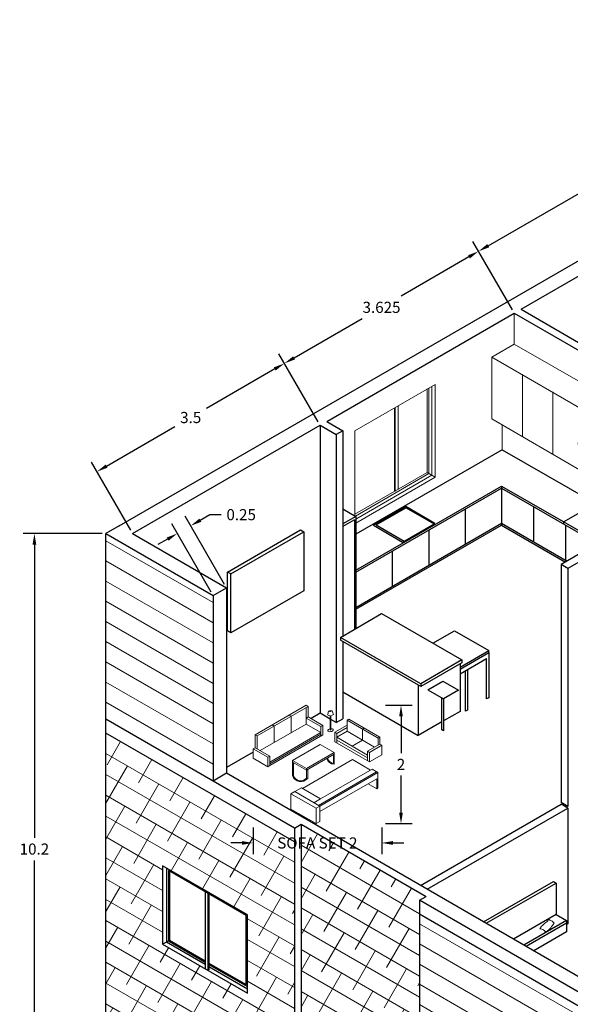
# Model space of a CAD drawing. Units: metres. Extents: x 14054 to 28215, y 4175 to 8383.
# Tile 2 of 6: x 14054.38 to 14063.29, y 4183.08 to 4199. Entities that reach past the tile are written whole.
import ezdxf

# ---------------------------------------------------------------- set-up
doc = ezdxf.new("R2010")
doc.units = ezdxf.units.M
for name, color, linetype, lineweight in [('A-ANNO-DIMS', 2, 'Continuous', 18), ('A-ANNO-NPLT', 9, 'Continuous', 13), ('A-ELEV-ISOM', 7, 'Continuous', 25), ('A-FURN', 8, 'Continuous', 13), ('A-GLAZ', 4, 'Continuous', 18), ('A-WALL-PATT', 8, 'Continuous', 13)]:
    doc.layers.add(name, color=color, linetype=linetype, lineweight=lineweight)
doc.styles.get("Standard").update_dxf_attribs({"font": 'arial.ttf'})
doc.dimstyles.get("Standard").update_dxf_attribs({"dimtxt": 0.18, "dimasz": 0.18, "dimexe": 0.18, "dimexo": 0.0625, "dimgap": 0.09, "dimtad": 0, "dimtih": 1, "dimtoh": 1, "dimdec": 4, "dimzin": 0, "dimdsep": 46, "dimtxsty": 'Standard', "dimcen": 0.09, "dimadec": 0, "dimazin": 0, "dimtfac": 1, "dimtdec": 4, "dimtofl": 0, "dimtmove": 0, "dimatfit": 3, "dimfxl": 1, "dimtolj": 1, "dimtzin": 0, "dimarcsym": 0})

# ---------------------------------------------------------------- blocks, each defined once
blk = doc.blocks.new('WINDOWS')
for p, q in [((14062.382, 4194.254), (14062.382, 4193.754)), ((14062.382, 4193.754), (14062.017, 4193.543)), ((14062.382, 4193.754), (14065.846, 4191.754)), ((14062.017, 4193.543), (14065.481, 4191.543)), ((14062.017, 4193.543), (14062.017, 4192.543)), ((14062.512, 4193.258), (14062.512, 4192.258)), ((14063.007, 4192.972), (14063.007, 4191.972)), ((14063.502, 4192.686), (14063.502, 4192.214)), ((14062.017, 4192.543), (14063.502, 4191.686)), ((14062.187, 4192.446), (14062.187, 4192.046)), ((14063.997, 4192.4), (14063.997, 4191.928)), ((14063.502, 4192.214), (14063.414, 4192.164)), ((14063.414, 4192.164), (14064.411, 4191.589)), ((14063.414, 4192.164), (14063.414, 4192.132)), ((14063.502, 4192.214), (14064.498, 4191.639)), ((14063.414, 4192.132), (14064.411, 4191.557)), ((14063.502, 4192.082), (14063.502, 4191.686)), ((14064.498, 4192.111), (14064.498, 4191.111)), ((14064.987, 4191.829), (14064.987, 4191.258)), ((14064.498, 4191.639), (14064.411, 4191.589)), ((14064.411, 4191.589), (14064.411, 4191.557)), ((14064.411, 4191.557), (14064.498, 4191.589)), ((14064.498, 4191.111), (14064.615, 4191.043))]:
    blk.add_line(p, q)
for p in [(14062.512, 4193.258), (14063.007, 4192.972), (14063.502, 4192.686), (14064.492, 4192.115), (14064.987, 4191.829)]:
    blk.add_point(p)
blk = doc.blocks.new('WINDOW')
for p, q in [((14059.806, 4192.353), (14061.105, 4193.103)), ((14061.105, 4193.103), (14061.105, 4191.603)), ((14060.975, 4193.028), (14060.975, 4191.678)), ((14061.002, 4193.043), (14061.002, 4191.663)), ((14061.047, 4193.069), (14061.047, 4191.637)), ((14060.445, 4192.722), (14060.445, 4191.384)), ((14060.456, 4192.728), (14060.456, 4191.378)), ((14060.505, 4192.756), (14060.505, 4191.406)), ((14059.806, 4190.976), (14059.806, 4192.353)), ((14060.975, 4191.678), (14059.806, 4191.003)), ((14060.975, 4191.678), (14061.105, 4191.603)), ((14061.002, 4191.663), (14059.815, 4190.971)), ((14061.047, 4191.637), (14059.821, 4190.923)), ((14061.105, 4191.603), (14059.821, 4190.861)), ((14060.456, 4191.378), (14060.445, 4191.384))]:
    blk.add_line(p, q)
blk = doc.blocks.new('SOFA SET')
for p, q in [((14050.583, 4183.453), (14052.129, 4184.345)), ((14050.646, 4183.417), (14052.188, 4184.311)), ((14052.129, 4184.345), (14052.188, 4184.311)), ((14052.129, 4183.775), (14052.129, 4184.277)), ((14052.188, 4183.991), (14052.188, 4184.311)), ((14052.841, 4184.171), (14052.866, 4184.172)), ((14052.841, 4184.171), (14052.841, 4184.156)), ((14052.866, 4184.172), (14052.866, 4184.158)), ((14051.674, 4184.013), (14051.614, 4184.048)), ((14051.674, 4184.013), (14051.674, 4183.512)), ((14052.129, 4183.957), (14052.188, 4183.991)), ((14052.572, 4183.701), (14052.129, 4183.957)), ((14052.631, 4183.735), (14052.188, 4183.991)), ((14052.851, 4183.602), (14052.851, 4184.028)), ((14052.868, 4183.603), (14052.868, 4184.029)), ((14053.361, 4183.896), (14053.411, 4183.925)), ((14054.298, 4183.355), (14053.361, 4183.896)), ((14053.361, 4183.896), (14053.361, 4183.56)), ((14054.348, 4183.384), (14053.411, 4183.925)), ((14052.129, 4183.775), (14050.741, 4182.974)), ((14051.16, 4183.715), (14051.099, 4183.75)), ((14051.16, 4183.715), (14051.16, 4183.216)), ((14052.129, 4183.775), (14052.572, 4183.519)), ((14052.572, 4183.701), (14052.631, 4183.735)), ((14052.572, 4183.416), (14052.572, 4183.701)), ((14052.572, 4183.622), (14052.572, 4183.416)), ((14052.631, 4183.735), (14052.631, 4183.45)), ((14052.989, 4183.528), (14053.361, 4183.743)), ((14053.048, 4183.494), (14053.361, 4183.675)), ((14053.048, 4183.379), (14053.361, 4183.56)), ((14053.361, 4183.56), (14054.193, 4183.079)), ((14053.83, 4183.626), (14053.879, 4183.654)), ((14053.83, 4183.289), (14053.83, 4183.626)), ((14050.583, 4183.064), (14050.583, 4183.453)), ((14050.583, 4183.453), (14050.646, 4183.417)), ((14050.646, 4183.028), (14050.646, 4183.417)), ((14051.027, 4182.627), (14052.572, 4183.519)), ((14052.572, 4183.469), (14051.027, 4182.577)), ((14051.027, 4182.524), (14052.631, 4183.45)), ((14052.572, 4183.416), (14052.631, 4183.45)), ((14052.989, 4183.528), (14052.989, 4183.243)), ((14052.989, 4183.528), (14053.048, 4183.494)), ((14053.048, 4183.494), (14053.048, 4183.209)), ((14053.048, 4183.379), (14053.98, 4182.841)), ((14053.048, 4183.292), (14053.98, 4182.754)), ((14053.83, 4183.289), (14053.516, 4183.109)), ((14054.298, 4183.355), (14054.348, 4183.384)), ((14054.298, 4183.355), (14054.298, 4183.14)), ((14054.348, 4183.169), (14054.348, 4183.384)), ((14050.524, 4183.03), (14050.583, 4183.064)), ((14050.968, 4182.775), (14050.524, 4183.03)), ((14050.524, 4182.746), (14050.524, 4183.03)), ((14051.027, 4182.808), (14050.583, 4183.064)), ((14051.717, 4182.68), (14052.549, 4183.161)), ((14052.549, 4183.161), (14052.968, 4182.919)), ((14052.989, 4183.243), (14054.039, 4182.637)), ((14053.98, 4182.956), (14054.348, 4183.169)), ((14054.039, 4182.922), (14054.406, 4183.135)), ((14054.348, 4183.169), (14054.406, 4183.135)), ((14054.406, 4183.135), (14054.406, 4182.85)), ((14050.524, 4182.746), (14050.968, 4182.49)), ((14050.968, 4182.775), (14051.027, 4182.808)), ((14050.968, 4182.49), (14050.968, 4182.775)), ((14051.027, 4182.808), (14051.027, 4182.524)), ((14051.717, 4182.68), (14052.136, 4182.438)), ((14051.717, 4182.68), (14051.717, 4182.629)), ((14052.014, 4181.835), (14053.522, 4182.706)), ((14052.968, 4182.919), (14052.136, 4182.438)), ((14052.968, 4182.868), (14052.136, 4182.387)), ((14052.95, 4182.857), (14052.95, 4182.587)), ((14052.968, 4182.919), (14052.968, 4182.868)), ((14052.968, 4182.868), (14052.968, 4182.571)), ((14054.07, 4182.389), (14053.522, 4182.706)), ((14053.98, 4182.956), (14053.98, 4182.671)), ((14053.98, 4182.956), (14054.039, 4182.922)), ((14054.039, 4182.922), (14054.039, 4182.637)), ((14054.039, 4182.637), (14054.406, 4182.85)), ((14050.968, 4182.49), (14051.027, 4182.524)), ((14051.717, 4182.629), (14052.136, 4182.387)), ((14051.717, 4182.629), (14051.717, 4182.222)), ((14051.747, 4182.612), (14051.747, 4182.23)), ((14052.136, 4182.438), (14052.136, 4182.387)), ((14052.136, 4182.387), (14052.136, 4182.145)), ((14052.173, 4182.408), (14052.173, 4182.138)), ((14052.563, 4181.519), (14054.115, 4182.415)), ((14054.115, 4182.415), (14054.295, 4182.311)), ((14052.498, 4181.322), (14054.253, 4182.335)), ((14052.54, 4181.297), (14054.295, 4182.311)), ((14054.259, 4182.128), (14052.54, 4181.136)), ((14054.259, 4181.827), (14054.259, 4182.128)), ((14054.295, 4182.311), (14054.295, 4181.848)), ((14051.982, 4181.854), (14051.78, 4181.737)), ((14051.982, 4181.854), (14052.563, 4181.519)), ((14054.259, 4181.827), (14053.998, 4181.977)), ((14054.295, 4181.848), (14054.259, 4181.827)), ((14051.669, 4181.673), (14051.78, 4181.737)), ((14052.43, 4181.234), (14051.669, 4181.673)), ((14051.669, 4181.673), (14051.669, 4181.21)), ((14052.54, 4181.297), (14051.78, 4181.737)), ((14052.563, 4181.519), (14052.36, 4181.401)), ((14052.43, 4180.771), (14051.669, 4181.21)), ((14052.54, 4181.297), (14052.43, 4181.234)), ((14052.43, 4181.234), (14052.43, 4180.771)), ((14052.54, 4181.297), (14052.54, 4180.835)), ((14052.54, 4180.835), (14052.43, 4180.771))]:
    blk.add_line(p, q)
for centre, radius, start, end in [((14051.304, 4184.571), 1.554, 340.4218, 344.7864), ((14052.864, 4184.075), 0.107, 65.1675, 123.9082), ((14052.847, 4184.288), 0.132, 251.1123, 297.9633), ((14053.99, 4184.575), 1.155, 200.4581, 206.1076), ((14052.85, 4184.184), 0.156, 238.6818, 311.6356), ((14052.859, 4183.606), 0.00924, 209.3503, 340.6112), ((14052.959, 4182.785), 0.215, 191.8594, 272.3236), ((14052.98, 4182.8), 0.215, 192.442, 261.974), ((14051.968, 4182.306), 0.265, 198.4938, 320.7512), ((14051.963, 4182.286), 0.224, 194.5089, 320.6289)]:
    blk.add_arc(centre, radius, start, end)
blk.add_ellipse((14052.863, 4183.591), major_axis=(0.0831, 0.0164), ratio=0.501593, start_param=1.613506, end_param=7.695336)
for p in [(14051.674, 4184.013), (14051.16, 4183.715)]:
    blk.add_point(p)
blk = doc.blocks.new('*D8')
at = {"layer": 'A-ANNO-DIMS', "color": 0, "lineweight": -2, "transparency": 16777216}
for p, q in [((14058.158, 4185.939), (14058.158, 4185.51)), ((14060.238, 4185.939), (14060.238, 4185.51)), ((14057.978, 4185.69), (14057.798, 4185.69)), ((14060.418, 4185.69), (14060.598, 4185.69))]:
    blk.add_line(p, q, dxfattribs=at)
at = {"layer": 'A-ANNO-DIMS', "color": 0, "transparency": 16777216}
for points in [[(14057.978, 4185.72), (14057.978, 4185.66), (14058.158, 4185.69)], [(14060.418, 4185.72), (14060.418, 4185.66), (14060.238, 4185.69)]]:
    blk.add_solid(points, dxfattribs=at)
at = {"layer": 'Defpoints', "color": 0, "transparency": 16777216}
for p in [(14058.158, 4186.002), (14060.238, 4186.002), (14060.238, 4185.69)]:
    blk.add_point(p, dxfattribs=at)
at = {"layer": 'A-ANNO-DIMS', "color": 0, "transparency": 16777216, "insert": (14059.198, 4185.69), "char_height": 0.18, "attachment_point": 5}
blk.add_mtext('\\A1;SOFA SET 2', dxfattribs=at)
blk = doc.blocks.new('*D9')
at = {"layer": 'A-ANNO-DIMS', "color": 0, "lineweight": -2, "transparency": 16777216}
for p, q in [((14060.3, 4187.916), (14060.73, 4187.916)), ((14060.55, 4187.736), (14060.55, 4187.14)), ((14060.55, 4186.182), (14060.55, 4186.779)), ((14060.3, 4186.002), (14060.73, 4186.002))]:
    blk.add_line(p, q, dxfattribs=at)
at = {"layer": 'A-ANNO-DIMS', "color": 0, "transparency": 16777216}
for points in [[(14060.52, 4187.736), (14060.58, 4187.736), (14060.55, 4187.916)], [(14060.52, 4186.182), (14060.58, 4186.182), (14060.55, 4186.002)]]:
    blk.add_solid(points, dxfattribs=at)
at = {"layer": 'Defpoints', "color": 0, "transparency": 16777216}
for p in [(14060.238, 4187.916), (14060.55, 4187.916), (14060.238, 4186.002)]:
    blk.add_point(p, dxfattribs=at)
at = {"layer": 'A-ANNO-DIMS', "color": 0, "transparency": 16777216, "insert": (14060.55, 4186.959), "char_height": 0.18, "attachment_point": 5}
blk.add_mtext('\\A1;2', dxfattribs=at)
blk = doc.blocks.new('*D12')
at = {"layer": 'A-ANNO-DIMS', "color": 0, "lineweight": -2, "transparency": 16777216}
for p, q in [((14055.716, 4190.691), (14054.443, 4190.691)), ((14054.623, 4190.511), (14054.623, 4185.773)), ((14054.623, 4180.671), (14054.623, 4185.409)), ((14055.716, 4180.491), (14054.443, 4180.491))]:
    blk.add_line(p, q, dxfattribs=at)
at = {"layer": 'A-ANNO-DIMS', "color": 0, "transparency": 16777216}
for points in [[(14054.593, 4190.511), (14054.653, 4190.511), (14054.623, 4190.691)], [(14054.593, 4180.671), (14054.653, 4180.671), (14054.623, 4180.491)]]:
    blk.add_solid(points, dxfattribs=at)
at = {"layer": 'Defpoints', "color": 0, "transparency": 16777216}
for p in [(14054.623, 4190.691), (14055.778, 4190.691), (14055.778, 4180.491)]:
    blk.add_point(p, dxfattribs=at)
at = {"layer": 'A-ANNO-DIMS', "color": 0, "transparency": 16777216, "insert": (14054.623, 4185.591), "char_height": 0.18, "attachment_point": 5}
blk.add_mtext('\\A1;10.2', dxfattribs=at)
blk = doc.blocks.new('*D70')
at = {"layer": 'A-ANNO-DIMS', "color": 0, "lineweight": -2, "transparency": 16777216}
for p, q in [((14059.211, 4192.495), (14058.575, 4193.597)), ((14058.509, 4193.352), (14057.404, 4192.713)), ((14055.79, 4191.782), (14056.895, 4192.42)), ((14056.18, 4190.745), (14055.544, 4191.847))]:
    blk.add_line(p, q, dxfattribs=at)
at = {"layer": 'A-ANNO-DIMS', "color": 0, "transparency": 16777216}
for points in [[(14058.494, 4193.377), (14058.524, 4193.326), (14058.665, 4193.442)], [(14055.775, 4191.807), (14055.805, 4191.756), (14055.634, 4191.692)]]:
    blk.add_solid(points, dxfattribs=at)
at = {"layer": 'Defpoints', "color": 0, "transparency": 16777216}
for p in [(14058.665, 4193.442), (14059.243, 4192.441), (14056.211, 4190.691)]:
    blk.add_point(p, dxfattribs=at)
at = {"layer": 'A-ANNO-DIMS', "color": 0, "transparency": 16777216, "insert": (14057.15, 4192.567), "char_height": 0.18, "attachment_point": 5}
blk.add_mtext('\\A1;3.5', dxfattribs=at)
blk = doc.blocks.new('*D71')
at = {"layer": 'A-ANNO-DIMS', "color": 0, "lineweight": -2, "transparency": 16777216}
for p, q in [((14062.351, 4194.308), (14061.714, 4195.41)), ((14061.649, 4195.164), (14060.55, 4194.53)), ((14058.821, 4193.532), (14059.92, 4194.166)), ((14059.211, 4192.495), (14058.575, 4193.597))]:
    blk.add_line(p, q, dxfattribs=at)
at = {"layer": 'A-ANNO-DIMS', "color": 0, "transparency": 16777216}
for points in [[(14061.634, 4195.19), (14061.664, 4195.138), (14061.804, 4195.254)], [(14058.806, 4193.557), (14058.836, 4193.506), (14058.665, 4193.442)]]:
    blk.add_solid(points, dxfattribs=at)
at = {"layer": 'Defpoints', "color": 0, "transparency": 16777216}
for p in [(14061.804, 4195.254), (14062.382, 4194.254), (14059.243, 4192.441)]:
    blk.add_point(p, dxfattribs=at)
at = {"layer": 'A-ANNO-DIMS', "color": 0, "transparency": 16777216, "insert": (14060.235, 4194.348), "char_height": 0.18, "attachment_point": 5}
blk.add_mtext('\\A1;3.625', dxfattribs=at)
blk = doc.blocks.new('*D72')
at = {"layer": 'A-ANNO-DIMS', "color": 0, "lineweight": -2, "transparency": 16777216}
for p, q in [((14068.564, 4197.895), (14067.928, 4198.997)), ((14067.862, 4198.752), (14065.226, 4197.23)), ((14061.96, 4195.344), (14064.596, 4196.866)), ((14062.351, 4194.308), (14061.714, 4195.41))]:
    blk.add_line(p, q, dxfattribs=at)
at = {"layer": 'A-ANNO-DIMS', "color": 0, "transparency": 16777216}
for points in [[(14067.847, 4198.777), (14067.877, 4198.726), (14068.018, 4198.842)], [(14061.945, 4195.37), (14061.975, 4195.318), (14061.804, 4195.254)]]:
    blk.add_solid(points, dxfattribs=at)
at = {"layer": 'Defpoints', "color": 0, "transparency": 16777216}
for p in [(14068.018, 4198.842), (14068.596, 4197.841), (14062.382, 4194.254)]:
    blk.add_point(p, dxfattribs=at)
at = {"layer": 'A-ANNO-DIMS', "color": 0, "transparency": 16777216, "insert": (14064.911, 4197.048), "char_height": 0.18, "attachment_point": 5}
blk.add_mtext('\\A1;7.175', dxfattribs=at)
blk = doc.blocks.new('*D76')
at = {"layer": 'A-ANNO-DIMS', "color": 0, "lineweight": -2, "transparency": 16777216}
for p, q in [((14057.696, 4189.87), (14057.06, 4190.972)), ((14057.305, 4190.907), (14057.461, 4190.997)), ((14057.461, 4190.997), (14057.641, 4190.997)), ((14057.479, 4189.745), (14056.843, 4190.847)), ((14056.777, 4190.602), (14056.621, 4190.512))]:
    blk.add_line(p, q, dxfattribs=at)
at = {"layer": 'A-ANNO-DIMS', "color": 0, "transparency": 16777216}
for points in [[(14057.29, 4190.932), (14057.32, 4190.881), (14057.15, 4190.817)], [(14056.762, 4190.627), (14056.792, 4190.576), (14056.933, 4190.692)]]:
    blk.add_solid(points, dxfattribs=at)
at = {"layer": 'Defpoints', "color": 0, "transparency": 16777216}
for p in [(14057.15, 4190.817), (14057.727, 4189.816), (14057.511, 4189.691)]:
    blk.add_point(p, dxfattribs=at)
at = {"layer": 'A-ANNO-DIMS', "color": 0, "transparency": 16777216, "insert": (14057.966, 4190.997), "char_height": 0.18, "attachment_point": 5}
blk.add_mtext('\\A1;0.25', dxfattribs=at)

msp = doc.modelspace()

# ---------------------------------------------------------------- hatches: boundary and pattern name
at = {"layer": 'A-WALL-PATT'}
h = msp.add_hatch(dxfattribs=at)
h.set_pattern_fill('ANSI31', color=256, scale=0.089, angle=105)
h.paths.add_polyline_path([(14057.5105, 4189.6913), (14055.7785, 4190.6913), (14055.7785, 4187.6913), (14057.5105, 4186.6913)])
h = msp.add_hatch(dxfattribs=at)
h.set_pattern_fill('ANSI38', color=256, scale=0.092, angle=105)
h.paths.add_polyline_path([(14055.7785, 4187.4672), (14055.7785, 4180.7413), (14058.8262, 4178.9816), (14058.8262, 4185.7075)])
h.paths.add_polyline_path([(14058.0676, 4184.5273), (14058.0676, 4183.2595), (14056.6953, 4184.0519), (14056.6953, 4185.3196)], flags=16)
h.paths.add_polyline_path([(14056.7604, 4184.0895), (14056.7893, 4184.1061), (14056.7893, 4185.2436), (14058.0488, 4184.5164), (14058.0488, 4183.401), (14057.4455, 4183.7494), (14057.4455, 4183.6399), (14057.4272, 4183.6293), (14057.4272, 4184.8753), (14057.3815, 4184.9017), (14057.3815, 4183.7309)], flags=0)
h.paths.add_polyline_path([(14063.5727, 4180.0812), (14062.8942, 4180.4729), (14061.5218, 4181.2653), (14060.8587, 4181.6535), (14060.8401, 4177.8243), (14063.5727, 4176.2413)])
h.paths.add_polyline_path([(14060.8494, 4184.7636), (14060.9576, 4184.8261), (14058.9345, 4185.9941), (14058.9345, 4178.9191), (14060.8494, 4177.8136)])
h.paths.add_polyline_path([(14060.7529, 4181.7978), (14060.7529, 4181.7242), (14060.7529, 4178.127), (14059.0613, 4179.1036), (14059.0613, 4182.7744)], flags=16)
h.paths.add_polyline_path([(14059.2399, 4179.1538), (14059.2399, 4182.5977), (14060.0427, 4182.1342), (14060.0427, 4178.6903)], flags=0)
h.paths.add_polyline_path([(14060.215, 4182.0347), (14060.7096, 4181.7492), (14060.7096, 4178.3053), (14060.215, 4178.5908)], flags=0)
edge = h.paths.add_edge_path(flags=0)
edge.add_ellipse((14059.9307, 4180.1763), major_axis=(-0.0333, 0.0192), ratio=0.8810932, start_angle=0, end_angle=360)
h = msp.add_hatch(dxfattribs=at)
h.set_pattern_fill('ANSI31', color=256, scale=0.089, angle=105)
h.paths.add_polyline_path([(14063.5727, 4182.9672), (14060.8494, 4184.5395), (14060.8494, 4181.6535), (14061.5218, 4181.2653), (14061.5218, 4182.533), (14062.8942, 4181.7407), (14062.8942, 4180.4729), (14063.5727, 4180.0812)])

# ---------------------------------------------------------------- linework, layer by layer
at = {"layer": 'A-ANNO-NPLT'}
for p in [(14061.5872, 4191.0845), (14062.6927, 4191.1262), (14060.9983, 4190.7445), (14063.2093, 4190.828), (14060.4095, 4190.4046)]:
    msp.add_point(p, dxfattribs=at)
at = {"layer": 'A-ELEV-ISOM'}
for p, q in [((14055.995, 4190.8163), (14068.5957, 4198.0913)), ((14062.4902, 4194.3163), (14068.5957, 4197.8413)), ((14059.3508, 4192.5038), (14062.3819, 4194.2538)), ((14062.3819, 4194.2538), (14065.9543, 4192.1913)), ((14062.4902, 4194.3163), (14065.9543, 4192.3163)), ((14059.3508, 4192.5038), (14059.6106, 4192.3538)), ((14056.2115, 4190.6913), (14059.2426, 4192.4413)), ((14059.2426, 4192.4413), (14059.5024, 4192.2913)), ((14059.2426, 4192.4413), (14059.2426, 4187.7856)), ((14059.6106, 4192.3538), (14059.5024, 4192.2913)), ((14059.6106, 4192.3538), (14059.6106, 4189.0365)), ((14059.5024, 4192.2913), (14059.5024, 4187.6356)), ((14062.1865, 4192.0456), (14059.821, 4190.6799)), ((14062.1865, 4192.0456), (14064.269, 4190.8433)), ((14065.846, 4191.7538), (14063.1397, 4190.1913)), ((14065.9543, 4191.6913), (14063.248, 4190.1288)), ((14059.8206, 4190.0646), (14062.1761, 4191.4245)), ((14059.821, 4190.1), (14062.1761, 4191.4597)), ((14062.1761, 4191.4597), (14063.7564, 4190.5473)), ((14062.1761, 4191.4597), (14062.1761, 4190.8279)), ((14062.1761, 4191.4245), (14063.7259, 4190.5297)), ((14059.6106, 4191.0887), (14059.821, 4190.9672)), ((14060.1036, 4190.8262), (14060.6263, 4191.128)), ((14060.1489, 4190.8324), (14060.6263, 4191.108)), ((14061.0972, 4190.8561), (14060.6263, 4191.128)), ((14060.6263, 4191.128), (14060.6263, 4191.108)), ((14061.0798, 4190.8461), (14060.6263, 4191.108)), ((14061.5872, 4191.0845), (14061.5872, 4190.517)), ((14062.6927, 4191.1262), (14062.6927, 4190.5587)), ((14063.1795, 4190.8803), (14063.6922, 4191.1763)), ((14059.821, 4190.9672), (14059.6106, 4190.8458)), ((14059.7965, 4190.9125), (14059.6106, 4190.8052)), ((14059.7965, 4190.9125), (14059.7965, 4189.1438)), ((14059.821, 4190.9672), (14059.821, 4190.9266)), ((14059.821, 4190.9266), (14059.821, 4189.158)), ((14063.1795, 4190.8803), (14063.1795, 4190.8451)), ((14055.995, 4190.8163), (14055.7785, 4190.6913)), ((14057.7473, 4190.0695), (14058.9236, 4190.7487)), ((14057.801, 4190.0385), (14058.9773, 4190.7177)), ((14058.9236, 4190.7487), (14058.9773, 4190.7177)), ((14058.9773, 4190.7177), (14058.9773, 4189.7668)), ((14059.8206, 4189.497), (14062.1761, 4190.857)), ((14059.8206, 4189.468), (14062.1761, 4190.8279)), ((14060.1036, 4190.8262), (14060.5745, 4190.5544)), ((14060.1489, 4190.8324), (14060.6025, 4190.5705)), ((14060.5745, 4190.5544), (14061.0972, 4190.8561)), ((14060.9983, 4190.7445), (14060.9983, 4190.177)), ((14062.1761, 4190.857), (14063.2344, 4190.2459)), ((14062.1761, 4190.8279), (14063.2093, 4190.2314)), ((14063.2093, 4190.828), (14063.2093, 4190.2604)), ((14055.7785, 4187.6913), (14055.7785, 4190.6913)), ((14055.7785, 4190.6913), (14057.5105, 4189.6913)), ((14056.2115, 4190.6913), (14057.727, 4189.8163)), ((14060.4095, 4190.4046), (14060.4095, 4189.837)), ((14063.248, 4190.1288), (14063.1397, 4190.1913)), ((14063.1397, 4190.1913), (14063.1397, 4186.3439)), ((14063.248, 4190.1288), (14063.248, 4186.2814)), ((14057.7473, 4189.1187), (14057.7473, 4190.0695)), ((14057.801, 4190.0385), (14057.7473, 4190.0695)), ((14057.801, 4189.0877), (14057.801, 4190.0385)), ((14057.5105, 4189.6913), (14057.727, 4189.8163)), ((14057.727, 4189.8163), (14057.727, 4186.8163)), ((14058.9773, 4189.7668), (14057.801, 4189.0877)), ((14057.5105, 4189.6913), (14057.5105, 4186.6913)), ((14059.5695, 4189.0128), (14060.2368, 4189.398)), ((14060.2368, 4189.398), (14061.5359, 4188.648)), ((14061.0656, 4188.9196), (14061.4129, 4189.1201)), ((14061.4129, 4189.1201), (14061.9689, 4188.7991)), ((14057.801, 4189.0877), (14057.7473, 4189.1187)), ((14060.8686, 4188.2628), (14059.5695, 4189.0128)), ((14059.5695, 4189.0128), (14059.5695, 4188.9684)), ((14060.8686, 4188.2184), (14059.5695, 4188.9684)), ((14059.6106, 4188.9447), (14059.6106, 4187.6981)), ((14061.5359, 4188.648), (14060.8686, 4188.2628)), ((14061.5042, 4188.5308), (14061.9689, 4188.7991)), ((14061.5042, 4188.4984), (14061.9689, 4188.7667)), ((14061.5042, 4188.4212), (14061.9347, 4188.6698)), ((14061.5359, 4188.648), (14061.5359, 4188.6037)), ((14061.9347, 4188.0171), (14061.9347, 4188.6698)), ((14061.9689, 4188.7667), (14061.9689, 4188.7991)), ((14061.9689, 4188.7667), (14061.9689, 4188.0368)), ((14061.5359, 4188.6037), (14060.8686, 4188.2184)), ((14061.5042, 4188.5854), (14061.5042, 4187.816)), ((14061.6253, 4188.4911), (14061.6253, 4187.8385)), ((14061.5919, 4187.8192), (14061.5919, 4188.4718)), ((14060.8289, 4188.2414), (14060.8289, 4187.4287)), ((14060.8686, 4188.2628), (14060.8686, 4188.2184)), ((14060.9839, 4188.1661), (14061.2266, 4188.3062)), ((14060.9839, 4188.1661), (14061.2379, 4188.0194)), ((14061.2266, 4188.3062), (14061.4807, 4188.1596)), ((14059.6106, 4188.1321), (14060.8289, 4187.4287)), ((14061.2086, 4187.5191), (14061.2086, 4188.0364)), ((14061.4807, 4188.1596), (14061.2379, 4188.0194)), ((14061.2379, 4188.0194), (14061.2379, 4187.5022)), ((14061.9689, 4188.0368), (14061.9347, 4188.0171)), ((14055.7785, 4180.4913), (14055.7785, 4187.6913)), ((14058.8262, 4185.9316), (14055.7785, 4187.6913)), ((14059.2426, 4187.7856), (14059.0949, 4187.7003)), ((14059.4045, 4187.6921), (14059.2426, 4187.7856)), ((14059.5024, 4187.6356), (14059.4135, 4187.6869)), ((14059.5024, 4187.6356), (14059.6106, 4187.6981)), ((14061.5042, 4187.816), (14061.2379, 4187.6633)), ((14061.6253, 4187.8385), (14061.5919, 4187.8192)), ((14061.2086, 4187.6465), (14060.8289, 4187.4287)), ((14058.8262, 4185.7075), (14055.7785, 4187.4672)), ((14061.2379, 4187.5022), (14061.2086, 4187.5191)), ((14058.1583, 4187.1596), (14057.727, 4186.9106)), ((14057.727, 4186.8163), (14057.5105, 4186.6913)), ((14063.572, 4183.4416), (14057.727, 4186.8163)), ((14060.8654, 4185.0043), (14063.1394, 4186.3172)), ((14060.974, 4184.9416), (14063.248, 4186.2545)), ((14063.248, 4186.2545), (14063.1394, 4186.3172)), ((14063.248, 4186.2814), (14063.1397, 4186.3439)), ((14063.248, 4186.2545), (14063.248, 4184.3824)), ((14058.8262, 4185.9316), (14058.9345, 4185.9941)), ((14058.9345, 4185.9941), (14060.9576, 4184.8261)), ((14058.9345, 4185.9941), (14058.9345, 4178.9191)), ((14058.8262, 4185.9316), (14058.8262, 4178.9816)), ((14058.0676, 4184.5273), (14056.6953, 4185.3196)), ((14056.6953, 4185.3196), (14056.6953, 4184.0519)), ((14056.7604, 4185.282), (14056.7604, 4184.0895)), ((14056.7893, 4185.2436), (14056.7893, 4184.1061)), ((14058.0488, 4184.5164), (14056.7893, 4185.2436)), ((14056.8084, 4185.2326), (14056.8084, 4184.1172)), ((14061.8851, 4184.4156), (14063.0139, 4185.0673)), ((14061.928, 4184.3908), (14063.0567, 4185.0425)), ((14063.0139, 4185.0673), (14063.0567, 4185.0425)), ((14063.0567, 4185.0425), (14063.0567, 4184.5326)), ((14057.3815, 4184.9017), (14057.3815, 4183.6557)), ((14057.4272, 4184.8753), (14057.4272, 4183.6293)), ((14057.4455, 4184.8647), (14057.4455, 4183.6399)), ((14060.8494, 4184.7636), (14060.9576, 4184.8261)), ((14063.5727, 4183.1913), (14060.8494, 4184.7636)), ((14060.8494, 4184.7636), (14060.8494, 4177.8136)), ((14058.0488, 4183.401), (14058.0488, 4184.5164)), ((14058.0676, 4183.2595), (14058.0676, 4184.5273)), ((14063.5727, 4182.9672), (14060.8494, 4184.5395)), ((14063.0567, 4184.5326), (14062.3696, 4184.1359)), ((14063.0567, 4184.5326), (14063.2254, 4184.4352)), ((14063.2254, 4184.4352), (14062.5383, 4184.0385)), ((14063.2254, 4184.3926), (14062.5752, 4184.0172)), ((14063.2254, 4184.4352), (14063.2254, 4184.2536)), ((14063.248, 4184.3824), (14063.2254, 4184.3693)), ((14063.2254, 4184.2536), (14062.6956, 4183.9477)), ((14056.6953, 4184.0519), (14056.8084, 4184.1172)), ((14056.6953, 4184.0519), (14058.0676, 4183.2595)), ((14056.7604, 4184.0895), (14057.3815, 4183.7309)), ((14056.7893, 4184.1061), (14057.3815, 4183.7643)), ((14056.8084, 4184.1172), (14057.3815, 4183.7863)), ((14057.4455, 4183.7494), (14058.0488, 4183.401)), ((14057.4455, 4183.7273), (14058.0676, 4183.3681)), ((14057.4272, 4183.6293), (14057.4455, 4183.6399)), ((14057.4455, 4183.6939), (14058.0676, 4183.3347))]:
    msp.add_line(p, q, dxfattribs=at)
at = {"layer": 'A-FURN'}
for points, knots in [([(14062.7945, 4184.3014), (14062.8006, 4184.3113), (14062.8187, 4184.3406), (14062.8603, 4184.3841), (14062.9169, 4184.4132), (14062.9318, 4184.448), (14062.9365, 4184.459)], [0, 0, 0, 0, 0.03482987, 0.10313679, 0.17946025, 0.21473211, 0.21473211, 0.21473211, 0.21473211]), ([(14062.9091, 4184.2572), (14062.9303, 4184.2777), (14062.9727, 4184.3189), (14063.0067, 4184.3672), (14063.0237, 4184.3914)], [0, 0, 0, 0, 0.08843034, 0.17682716, 0.17682716, 0.17682716, 0.17682716]), ([(14062.9365, 4184.459), (14062.9508, 4184.4486), (14062.9724, 4184.4329), (14063.0079, 4184.4182), (14063.0182, 4184.4008), (14063.0237, 4184.3914)], [0, 0, 0, 0, 0.05304895, 0.08028585, 0.1118807, 0.1118807, 0.1118807, 0.1118807]), ([(14062.7945, 4184.3014), (14062.8181, 4184.3006), (14062.8562, 4184.2992), (14062.8802, 4184.2453), (14062.9015, 4184.2591), (14062.9081, 4184.2574), (14062.9091, 4184.2572)], [0, 0, 0, 0, 0.06697653, 0.10836817, 0.12560013, 0.12860318, 0.12860318, 0.12860318, 0.12860318])]:
    msp.add_open_spline(points, degree=3, knots=knots, dxfattribs=at)

# ---------------------------------------------------------------- block references
at = {"layer": 'A-FURN', "xscale": 0.5356833887185518, "yscale": 0.5356833887185518, "zscale": 0.5356833887185518}
msp.add_blockref('SOFA SET', (6531.5257, 1946.4323), dxfattribs=at)
at = {"layer": 'A-GLAZ'}
for name in ['WINDOWS', 'WINDOW']:
    msp.add_blockref(name, (0, 0), dxfattribs=at)

# ---------------------------------------------------------------- dimensions: what is measured, and where the dimension line sits
at = {"layer": 'A-ANNO-DIMS'}
for base, p1, p2, angle, override, picture, middle in [((14068.0182, 4198.8415), (14062.3819, 4194.2538), (14068.5957, 4197.8413), 30, {"dimdec": 3, "dimlfac": 1, "dimrnd": 0, "dimzin": 0, "dimdsep": 46, "dimlunit": 2}, '*D72', (14064.9113, 4197.0478)), ((14061.8044, 4195.254), (14059.2426, 4192.4413), (14062.3819, 4194.2538), 30, {"dimdec": 3, "dimlfac": 1, "dimrnd": 0, "dimzin": 0, "dimdsep": 46, "dimlunit": 2}, '*D71', (14060.2348, 4194.3478)), ((14058.6651, 4193.4415), (14056.2115, 4190.6913), (14059.2426, 4192.4413), 30, {"dimdec": 1, "dimlfac": 1, "dimrnd": 0, "dimzin": 0, "dimdsep": 46, "dimlunit": 2}, '*D70', (14057.1495, 4192.5665)), ((14057.1495, 4190.8165), (14057.5105, 4189.6913), (14057.727, 4189.8163), 30, {"dimdec": 2, "dimlfac": 1, "dimrnd": 0, "dimzin": 0, "dimdsep": 46, "dimlunit": 2}, '*D76', (14057.9658, 4190.9965)), ((14054.6235, 4190.6913), (14055.7785, 4180.4913), (14055.7785, 4190.6913), 90, {"dimdec": 1, "dimlfac": 1, "dimrnd": 0, "dimzin": 0, "dimdsep": 46, "dimlunit": 2}, '*D12', (14054.6235, 4185.5913)), ((14060.5497, 4187.9165), (14060.2378, 4186.002), (14060.2378, 4187.9165), 90, {"dimdec": 0, "dimlfac": 1, "dimrnd": 0, "dimzin": 0, "dimdsep": 46, "dimlunit": 2}, '*D9', (14060.5497, 4186.9592))]:
    dim = msp.add_linear_dim(base=base, p1=p1, p2=p2, angle=angle, dimstyle='Standard', override=override, dxfattribs=at)
    dim.commit()
    dim.dimension.update_dxf_attribs({"geometry": picture, "text_midpoint": middle})
dim = msp.add_linear_dim(base=(14060.2378, 4185.6901), p1=(14058.1583, 4186.002), p2=(14060.2378, 4186.002), text='SOFA SET <>', dimstyle='Standard', override={"dimdec": 0, "dimlfac": 1, "dimrnd": 0, "dimzin": 0, "dimdsep": 46, "dimlunit": 2}, dxfattribs=at)
dim.commit()
dim.dimension.update_dxf_attribs({"geometry": '*D8', "text_midpoint": (14059.1981, 4185.6901)})

doc.saveas('drawing.dxf')
